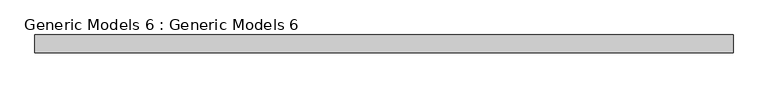
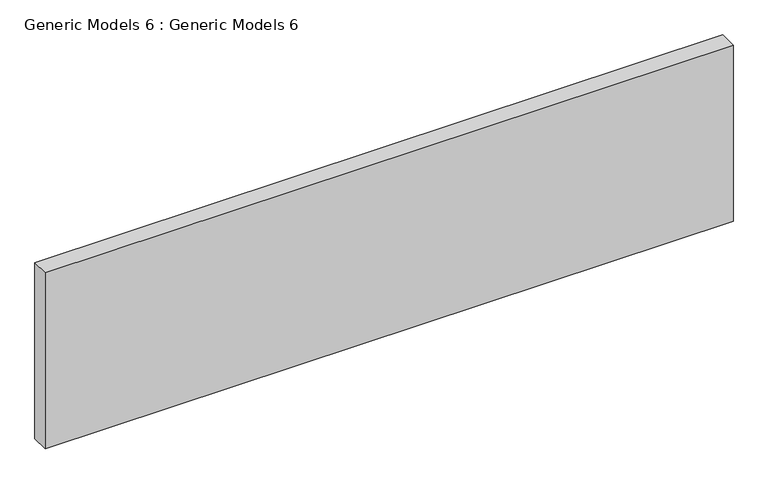
"""IFC4 building model written with IfcOpenShell, lengths in millimetres: proxy geometry, Generic Models 6 : Generic Models 6."""

from ifc_helpers import new_model, si_unit, frame, origin, place, context, project, spatial, polyline, outline, extrude, source, transform, mapped, element, save


def generic_models_6_generic_models_6_46bcb04b(model_context):
    return source(origin(), model_context, "Body", "SweptSolid", [
        extrude(outline(polyline([(-17832.2537599, -14261.7752569), (-17832.2537599, -14134.7752569), (-12874.4414575, -14134.7752569), (-12874.4414575, -14261.7752569), (-17832.2537599, -14261.7752569)])), frame((0.0, 0.0, 9448.8), z_axis=(0.0, 0.0, 1.0), x_axis=(1.0, 0.0, 0.0)), (0.0, 0.0, 1.0), 1341.7282636),
    ])


if __name__ == "__main__":
    model = new_model("IFC4")
    model_context = context("Model", 3, world=origin())
    ifc_project = project(units=[si_unit("LENGTHUNIT", "METRE", prefix="MILLI")], contexts=[model_context])
    site = spatial("IfcSite", under=ifc_project)
    building = spatial("IfcBuilding", under=site)
    placement = place(None, origin())
    generic_models_6_generic_models_6_shape = generic_models_6_generic_models_6_46bcb04b(model_context)
    element("IfcBuildingElementProxy", 1, Name="Generic Models 6 : Generic Models 6", ObjectType="Generic Models 6 : Generic Models 6", at=placement, inside=building, context=model_context, shape_type="MappedRepresentation", body=[
        mapped(generic_models_6_generic_models_6_shape, transform((0.0, 0.0, 0.0), x_axis=(1.0, 0.0, 0.0), y_axis=(0.0, 1.0, 0.0), z_axis=(0.0, 0.0, 1.0))),
    ])
    save(model, "model.ifc")
